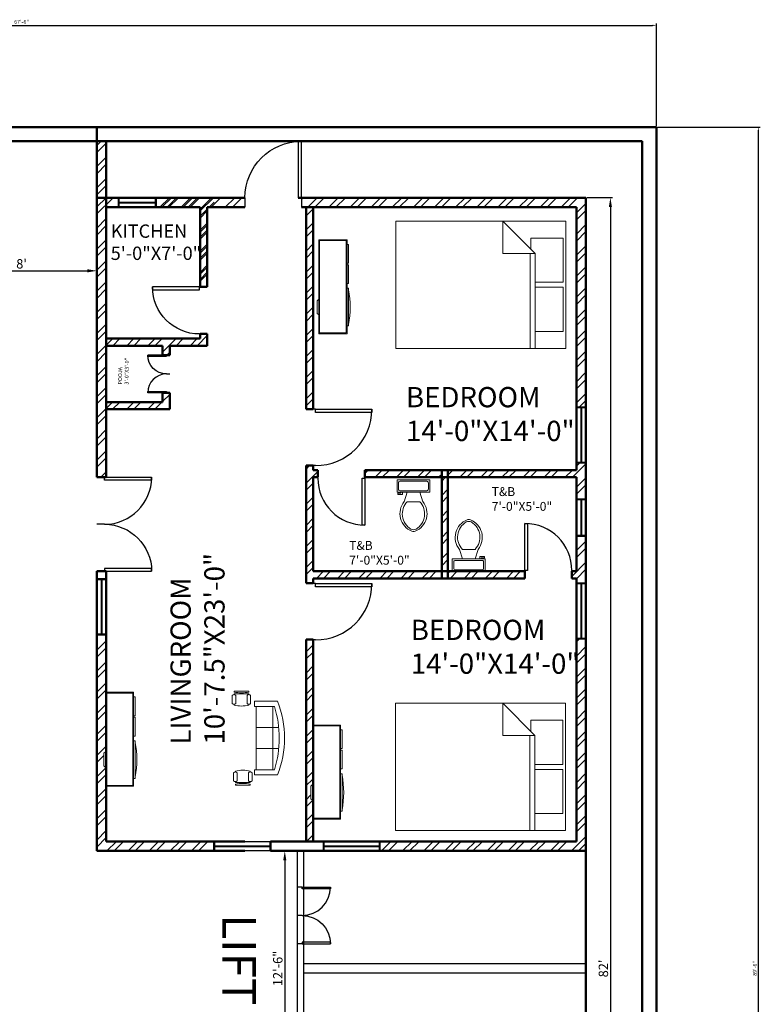
# Model space of a CAD drawing. Units: inches. Extents: x -12550 to 6516, y 1273 to 18700.
# Tile 19 of 19: x 6043 to 6516, y 1958 to 2587. Entities that reach past the tile are written whole.
import ezdxf

# ---------------------------------------------------------------- set-up
doc = ezdxf.new("R2010")
doc.units = ezdxf.units.IN
for name, color, linetype, lineweight in [('A-ANNO-DIMS', 2, 'Continuous', 18), ('A-AREA-IDEN', 1, 'Continuous', 18), ('A-DOOR', 5, 'Continuous', 25), ('A-EQPM', 4, 'Continuous', 25), ('A-FURN', 8, 'Continuous', 18), ('A-GLAZ', 3, 'Continuous', 25), ('A-WALL', 7, 'Continuous', 50), ('A-WALL-PATT', 8, 'Continuous', 13)]:
    doc.layers.add(name, color=color, linetype=linetype, lineweight=lineweight)
doc.styles.get("Standard").update_dxf_attribs({"font": 'arial.ttf'})
doc.dimstyles.new('ISO-25', dxfattribs={"dimtxt": 2.5, "dimasz": 2.5, "dimexe": 1.25, "dimexo": 0.625, "dimtad": 1, "dimlunit": 4, "dimtxsty": 'Standard', "dimcen": 2.5, "dimadec": 0, "dimazin": 0, "dimtfac": 1, "dimtmove": 0, "dimatfit": 3, "dimfxl": 1, "dimarcsym": 0})
pattern_1 = [(45, (3666.851, 0), (-6.735192, 6.735192), []), (45, (3671.341, 0), (-6.735192, 6.735192), [])]
pattern_2 = [(45, (3666.851, 567), (-6.735192, 6.735192), []), (45, (3671.341, 567), (-6.735192, 6.735192), [])]

# ---------------------------------------------------------------- blocks, each defined once
blk = doc.blocks.new('*U2')
for p, q in [((0, 0), (0, -5)), ((30, 0), (30, -5))]:
    blk.add_line(p, q)
blk.add_lwpolyline([(0, 0), (0, 30), (1.75, 30), (1.75, 0)], close=True)
blk.add_arc((0, 0), 30, 0, 90)
blk = doc.blocks.new('Bed - Queen')
for p, q in [((0, -80.00003), (0, 0)), ((0, 0), (59.99999, 0)), ((59.99999, 0), (59.99999, -80.00003)), ((7.99999, -1.2), (28.79998, -1.2)), ((7.99999, -14.4), (7.99999, -1.2)), ((28.79998, -1.2), (28.79998, -14.4)), ((31.19999, -1.2), (51.99999, -1.2)), ((31.19999, -14.4), (31.19999, -1.2)), ((51.99999, -1.2), (51.99999, -16.4)), ((0, -14.4), (44.8, -14.4)), ((44.8, -16.8), (0, -16.8)), ((59.99999, -29.6), (44.8, -14.4)), ((44.8, -14.4), (44.8, -29.6)), ((51.99999, -16.4), (46.79936, -16.4)), ((44.8, -29.6), (59.99999, -29.6)), ((59.99999, -80.00003), (0, -80.00003))]:
    blk.add_line(p, q)
blk = doc.blocks.new('Toilet - top')
for p, q in [((9.5, -6), (9.5, -2)), ((-10, -8.5), (-8, -8.5)), ((-10, -9.5), (-10, -8.5)), ((-7, -9.5), (-10, -9.5)), ((-8, -8.5), (-8, -8)), ((-7, -8), (-7, -9.5)), ((-4, -8), (-6, -14)), ((4, -8), (6, -14)), ((4, -14), (-4, -14))]:
    blk.add_line(p, q)
blk.add_lwpolyline([(10.5, -8), (10.5, 0), (-10.5, 0), (-10.5, -8)], close=True)
for points in [[(-9.5, -2), (-9.5, -6)], [(8.5, -1), (-8.5, -1)], [(-8.5, -7), (8.5, -7)]]:
    blk.add_lwpolyline(points)
for centre, radius, start, end in [((-8.62, -1.88), 0.884, 81.8699, 188.1301), ((-8.62, -6.12), 0.884, 171.8699, 278.1301), ((8.62, -1.88), 0.884, 351.8699, 98.1301), ((8.62, -6.12), 0.884, 261.8699, 8.1301), ((3.52, -21.58), 12.17, 141.46911, 247.97143), ((4.2, -21.82), 11.33, 136.36773, 238.94682), ((-3.52, -21.58), 12.17, 292.02843, 38.53071), ((-4.2, -21.82), 11.33, 301.05301, 43.63209), ((0, -27.88), 4, 245.73182, 294.26817), ((0, -29), 4, 254.86053, 285.13947)]:
    blk.add_arc(centre, radius, start, end)
blk = doc.blocks.new('Entertainment Center')
for p, q in [((-4, 0), (-5, -1)), ((4, 0), (-4, 0)), ((5, -1), (4, 0)), ((-17, -19), (-17, -1)), ((-17, -1), (43, -1)), ((-16.5, -18.5), (-16.5, -1.5)), ((-16.5, -1.5), (42.5, -1.5)), ((42.5, -1.5), (42.5, -18.5)), ((43, -1), (43, -19)), ((42.5, -18.5), (-16.5, -18.5)), ((43, -19), (-17, -19)), ((-12, -20), (-12, -19)), ((12, -20), (-12, -20)), ((12, -19), (12, -20)), ((15, -20), (15, -19)), ((27, -20), (15, -20)), ((27, -19), (27, -20)), ((28, -20), (28, -19)), ((40, -20), (28, -20)), ((40, -19), (40, -20))]:
    blk.add_line(p, q)
blk.add_arc((0, 40), 61, 259.6111, 280.3889)
blk = doc.blocks.new('Sofa - Roundback 7 ft.')
for p, q in [((-12.00002, -32.4421), (-12.00003, -6.5971)), ((11.99997, -32.4421), (11.99998, -6.5971)), ((-36.000027, -34), (-36.000027, -11.4696)), ((-35.999844, -13.3819), (35.9998, -13.3819)), ((35.99998, -34), (35.99998, -11.4696)), ((-36.000027, -32.4421), (35.99998, -32.4421))]:
    blk.add_line(p, q)
for points in [[(-36.000027, -34), (-42.000027, -34), (-42.000027, -8)], [(41.99998, -8), (41.99998, -34), (35.99998, -34)]]:
    blk.add_lwpolyline(points)
for centre, radius, start, end in [((0, -114.25), 114.25, 68.43141, 111.5686), ((-0.00001, -127.1968), 121.1968, 72.72033, 107.2797)]:
    blk.add_arc(centre, radius, start, end)
blk = doc.blocks.new('Chair - Desk')
for p, q in [((-8.5, 0), (-8.5, -1)), ((-8.5, 0), (8.5, 0)), ((8.5, 0), (8.5, -1)), ((-10.5, -5), (-10.5, -14)), ((-8.5, -3), (-8.5, -4)), ((-8.5, -3), (8.5, -3)), ((-6.5, -14), (-6.5, -5)), ((-2, -3), (-2, -1.9355)), ((2, -1.9576), (2, -3)), ((6.5, -5), (6.5, -14)), ((8.5, -3), (8.5, -4)), ((10.5, -14), (10.5, -5)), ((-8.5, -15), (-8.5, -16)), ((8.5, -15), (8.5, -16))]:
    blk.add_line(p, q)
for centre, radius, start, end in [((-8.5, -6.5), 2.5, 36.8699, 143.1301), ((0, 34.625), 36.625, 256.5803, 283.4197), ((8.5, -6.5), 2.5, 36.8699, 143.1301), ((-8.5, -12.5), 2.5, 216.8699, 323.1301), ((0, 19.625), 36.625, 256.5803, 283.4197), ((8.5, -12.5), 2.5, 216.8699, 323.1301)]:
    blk.add_arc(centre, radius, start, end)
blk = doc.blocks.new('*D52')
at = {"layer": 'A-ANNO-DIMS', "color": 0, "lineweight": -2, "transparency": 16777216}
for p, q in [((6219.91, 2056.25), (6211.2, 2056.25)), ((6212.45, 2050.25), (6212.45, 1912.25)), ((6219.91, 1906.25), (6211.2, 1906.25))]:
    blk.add_line(p, q, dxfattribs=at)
at = {"layer": 'A-ANNO-DIMS', "color": 0, "transparency": 16777216}
for points in [[(6211.45, 2050.25), (6213.45, 2050.25), (6212.45, 2056.25)], [(6211.45, 1912.25), (6213.45, 1912.25), (6212.45, 1906.25)]]:
    blk.add_solid(points, dxfattribs=at)
at = {"layer": 'Defpoints', "color": 0, "transparency": 16777216}
for p in [(6220.54, 2056.25), (6212.45, 1906.25), (6220.54, 1906.25)]:
    blk.add_point(p, dxfattribs=at)
at = {"layer": 'A-ANNO-DIMS', "color": 0, "transparency": 16777216, "insert": (6208.76, 1981.25), "char_height": 6, "attachment_point": 5, "rotation": 90}
blk.add_mtext('12\'-6"', dxfattribs=at)
blk = doc.blocks.new('*D54')
at = {"layer": 'A-ANNO-DIMS', "color": 0, "lineweight": -2, "transparency": 16777216}
for p, q in [((6405.16, 2473.25), (6421.41, 2473.25)), ((6420.16, 2467.25), (6420.16, 1495.25)), ((6405.16, 1489.25), (6421.41, 1489.25))]:
    blk.add_line(p, q, dxfattribs=at)
at = {"layer": 'A-ANNO-DIMS', "color": 0, "transparency": 16777216}
for points in [[(6419.16, 2467.25), (6421.16, 2467.25), (6420.16, 2473.25)], [(6419.16, 1495.25), (6421.16, 1495.25), (6420.16, 1489.25)]]:
    blk.add_solid(points, dxfattribs=at)
at = {"layer": 'Defpoints', "color": 0, "transparency": 16777216}
for p in [(6404.54, 2473.25), (6404.54, 1489.25), (6420.16, 1489.25)]:
    blk.add_point(p, dxfattribs=at)
at = {"layer": 'A-ANNO-DIMS', "color": 0, "transparency": 16777216, "insert": (6416.47, 1981.25), "char_height": 6, "attachment_point": 5, "rotation": 90}
blk.add_mtext("82'", dxfattribs=at)
blk = doc.blocks.new('*D51')
at = {"layer": 'A-ANNO-DIMS', "color": 0, "lineweight": -2, "transparency": 16777216}
for p, q in [((5996.54, 2407.12), (5996.54, 2427.81)), ((6002.54, 2426.56), (6086.54, 2426.56)), ((6092.54, 2407.12), (6092.54, 2427.81))]:
    blk.add_line(p, q, dxfattribs=at)
at = {"layer": 'A-ANNO-DIMS', "color": 0, "transparency": 16777216}
for points in [[(6002.54, 2427.56), (6002.54, 2425.56), (5996.54, 2426.56)], [(6086.54, 2427.56), (6086.54, 2425.56), (6092.54, 2426.56)]]:
    blk.add_solid(points, dxfattribs=at)
at = {"layer": 'Defpoints', "color": 0, "transparency": 16777216}
for p in [(6092.54, 2426.56), (5996.54, 2406.5), (6092.54, 2406.5)]:
    blk.add_point(p, dxfattribs=at)
at = {"layer": 'A-ANNO-DIMS', "color": 0, "transparency": 16777216, "insert": (6044.54, 2430.25), "char_height": 6, "attachment_point": 5}
blk.add_mtext("8'", dxfattribs=at)
blk = doc.blocks.new('WIN-3FT')
for p, q in [((0, 0), (0, 6)), ((0, 6), (36.02, 6)), ((36.02, 0), (0, 0)), ((0.5, 0), (0.5, 6)), ((35.52, 3.2), (0.5, 3.2)), ((35.52, 2.8), (0.5, 2.8)), ((35.52, 6), (35.52, 0)), ((36.02, 6), (36.02, 0))]:
    blk.add_line(p, q)
blk = doc.blocks.new('WIN-2FT')
for p, q in [((0, 0), (0, 24.02)), ((0, 24.02), (6, 24.02)), ((0, 23.52), (6, 23.52)), ((2.8, 0.5), (2.8, 23.52)), ((3.2, 0.5), (3.2, 23.52)), ((6, 24.02), (6, 0)), ((6, 0.5), (0, 0.5)), ((6, 0), (0, 0))]:
    blk.add_line(p, q)
blk = doc.blocks.new('*D121')
at = {"layer": 'A-ANNO-DIMS', "color": 0, "lineweight": -2, "transparency": 16777216}
for p, q in [((5639.54, 2518.87), (5639.54, 2584.5)), ((5642.04, 2583.25), (6447.04, 2583.25)), ((6449.54, 2518.87), (6449.54, 2584.5))]:
    blk.add_line(p, q, dxfattribs=at)
at = {"layer": 'A-ANNO-DIMS', "color": 0, "transparency": 16777216}
for points in [[(5642.04, 2583.66), (5642.04, 2582.83), (5639.54, 2583.25)], [(6447.04, 2583.66), (6447.04, 2582.83), (6449.54, 2583.25)]]:
    blk.add_solid(points, dxfattribs=at)
at = {"layer": 'Defpoints', "color": 0, "transparency": 16777216}
for p in [(6449.54, 2583.25), (5639.54, 2518.25), (6449.54, 2518.25)]:
    blk.add_point(p, dxfattribs=at)
at = {"layer": 'A-ANNO-DIMS', "color": 0, "transparency": 16777216, "insert": (6044.54, 2585.15), "char_height": 2.5, "attachment_point": 5}
blk.add_mtext('67\'-6"', dxfattribs=at)
blk = doc.blocks.new('*D122')
at = {"layer": 'A-ANNO-DIMS', "color": 0, "lineweight": -2, "transparency": 16777216}
for p, q in [((6450.16, 2518.25), (6515.79, 2518.25)), ((6514.54, 1446.75), (6514.54, 2515.75)), ((6450.16, 1444.25), (6515.79, 1444.25))]:
    blk.add_line(p, q, dxfattribs=at)
at = {"layer": 'A-ANNO-DIMS', "color": 0, "transparency": 16777216}
for points in [[(6514.12, 2515.75), (6514.96, 2515.75), (6514.54, 2518.25)], [(6514.12, 1446.75), (6514.96, 1446.75), (6514.54, 1444.25)]]:
    blk.add_solid(points, dxfattribs=at)
at = {"layer": 'Defpoints', "color": 0, "transparency": 16777216}
for p in [(6449.54, 2518.25), (6514.54, 2518.25), (6449.54, 1444.25)]:
    blk.add_point(p, dxfattribs=at)
at = {"layer": 'A-ANNO-DIMS', "color": 0, "transparency": 16777216, "insert": (6512.64, 1981.25), "char_height": 2.5, "attachment_point": 5, "rotation": 90}
blk.add_mtext('89\'-6"', dxfattribs=at)

msp = doc.modelspace()

# ---------------------------------------------------------------- hatches: boundary and pattern name
at = {"layer": 'A-WALL-PATT'}
h = msp.add_hatch(dxfattribs=at)
h.set_pattern_fill('ANSI32', color=256)
h.set_pattern_definition(pattern_1)
h.paths.add_polyline_path([(6098.54, 2509.247), (6092.54, 2509.247), (6092.54, 2473.247), (6098.54, 2473.247)])
h = msp.add_hatch(dxfattribs=at)
h.set_pattern_fill('ANSI32', color=256)
h.set_pattern_definition(pattern_2)
h.paths.add_polyline_path([(6106.297, 2473.247), (6092.54, 2473.247), (6092.54, 2294.747), (6097.54, 2294.747), (6098.54, 2294.747), (6098.54, 2467.247), (6106.297, 2467.247)])
h = msp.add_hatch(dxfattribs=at)
h.set_pattern_fill('ANSI32', color=256)
h.set_pattern_definition(pattern_1)
h.paths.add_polyline_path([(6130.314, 2473.247), (6130.314, 2467.247), (6158.54, 2467.247), (6158.54, 2416.247), (6163.04, 2416.247), (6163.04, 2467.247), (6187.04, 2467.247), (6187.04, 2473.247)])
h = msp.add_hatch(dxfattribs=at)
h.set_pattern_fill('ANSI32', color=256)
h.set_pattern_definition(pattern_2)
h.paths.add_polyline_path([(6167.378, 2473.247), (6130.314, 2473.247), (6130.314, 2467.247), (6158.54, 2467.247), (6158.54, 2416.247), (6163.04, 2416.247), (6163.04, 2467.247), (6167.378, 2467.247)])
h = msp.add_hatch(dxfattribs=at)
h.set_pattern_fill('ANSI32', color=256)
h.set_pattern_definition(pattern_2)
h.paths.add_polyline_path([(6223.04, 2473.247), (6223.04, 2467.247), (6398.54, 2467.247), (6398.54, 2339.747), (6404.54, 2339.747), (6404.54, 2473.247)])
h = msp.add_hatch(dxfattribs=at)
h.set_pattern_fill('ANSI32', color=256)
h.set_pattern_definition(pattern_2)
h.paths.add_polyline_path([(6230.54, 2467.247), (6226.04, 2467.247), (6226.04, 2338.247), (6230.54, 2338.247)])
h = msp.add_hatch(dxfattribs=at)
h.set_pattern_fill('ANSI32', color=256)
h.set_pattern_definition(pattern_2)
h.paths.add_polyline_path([(6163.04, 2386.247), (6158.54, 2386.247), (6158.54, 2383.247), (6098.54, 2383.247), (6098.54, 2378.747), (6134.54, 2378.747), (6134.54, 2372.747), (6137.04, 2372.747), (6139.04, 2372.747), (6139.04, 2378.747), (6163.04, 2378.747)])
h = msp.add_hatch(dxfattribs=at)
h.set_pattern_fill('ANSI32', color=256)
h.set_pattern_definition(pattern_2)
h.paths.add_polyline_path([(6139.04, 2348.747), (6137.04, 2348.747), (6134.54, 2348.747), (6134.54, 2342.747), (6098.54, 2342.747), (6098.54, 2338.247), (6139.04, 2338.247)])
h = msp.add_hatch(dxfattribs=at)
h.set_pattern_fill('ANSI32', color=256)
h.set_pattern_definition(pattern_2)
h.paths.add_polyline_path([(6230.54, 2294.747), (6233.54, 2294.747), (6233.54, 2299.247), (6230.54, 2299.247), (6230.54, 2302.247), (6226.04, 2302.247), (6226.04, 2227.247), (6230.54, 2227.247), (6230.54, 2230.247), (6233.492, 2230.247), (6312.54, 2230.247), (6312.54, 2234.747), (6233.492, 2234.747), (6230.54, 2234.747)])
h = msp.add_hatch(dxfattribs=at)
h.set_pattern_fill('ANSI32', color=256)
h.set_pattern_definition(pattern_2)
h.paths.add_polyline_path([(6404.54, 2303.73), (6398.54, 2303.73), (6398.54, 2299.247), (6395.54, 2299.247), (6316.54, 2299.247), (6316.54, 2294.747), (6395.54, 2294.747), (6398.54, 2294.747), (6398.54, 2281.042), (6404.54, 2281.042)])
h = msp.add_hatch(dxfattribs=at)
h.set_pattern_fill('ANSI32', color=256)
h.set_pattern_definition(pattern_2)
h.paths.add_polyline_path([(6312.54, 2299.247), (6263.54, 2299.247), (6263.54, 2294.747), (6312.54, 2294.747)], flags=17)
h = msp.add_hatch(dxfattribs=at)
h.set_pattern_fill('ANSI32', color=256)
h.set_pattern_definition(pattern_2)
h.paths.add_polyline_path([(6316.54, 2294.747), (6312.54, 2294.747), (6312.54, 2234.747), (6316.54, 2234.747)])
h = msp.add_hatch(dxfattribs=at)
h.set_pattern_fill('ANSI32', color=256)
h.set_pattern_definition(pattern_2)
h.paths.add_polyline_path([(6404.54, 2257.024), (6398.54, 2257.024), (6398.54, 2234.747), (6395.54, 2234.747), (6395.54, 2230.247), (6398.54, 2230.247), (6398.54, 2227.369), (6404.54, 2227.369)])
h = msp.add_hatch(dxfattribs=at)
h.set_pattern_fill('ANSI32', color=256)
h.set_pattern_definition(pattern_2)
h.paths.add_polyline_path([(6365.54, 2234.747), (6316.54, 2234.747), (6316.54, 2230.247), (6365.54, 2230.247)])
h = msp.add_hatch(dxfattribs=at)
h.set_pattern_fill('ANSI32', color=256)
h.set_pattern_definition(pattern_2)
h.paths.add_polyline_path([(6167.378, 2056.247), (6167.378, 2062.247), (6098.54, 2062.247), (6098.54, 2097.559), (6098.04, 2097.559), (6098.04, 2109.559), (6097.04, 2110.559), (6097.04, 2118.559), (6098.04, 2119.559), (6098.04, 2157.559), (6098.54, 2157.559), (6098.54, 2194.032), (6092.54, 2194.032), (6092.54, 2056.247)])
h = msp.add_hatch(dxfattribs=at)
h.set_pattern_fill('ANSI32', color=256)
h.set_pattern_definition(pattern_2)
h.paths.add_polyline_path([(6226.04, 2190.947), (6226.04, 2062.247), (6230.54, 2062.247), (6230.54, 2076.575), (6230.04, 2076.575), (6230.04, 2088.575), (6229.04, 2089.575), (6229.04, 2097.575), (6230.04, 2098.575), (6230.04, 2136.575), (6230.537, 2190.947)])
h = msp.add_hatch(dxfattribs=at)
h.set_pattern_fill('ANSI32', color=256)
h.set_pattern_definition(pattern_2)
h.paths.add_polyline_path([(6404.54, 2191.352), (6398.54, 2191.352), (6398.54, 2062.247), (6273.126, 2062.247), (6273.126, 2056.247), (6404.54, 2056.247)])

# ---------------------------------------------------------------- linework, layer by layer
at = {"layer": 'A-EQPM'}
for p, q in [((6220.54, 1906.247), (6220.54, 2056.247)), ((6404.54, 2056.247), (6220.54, 2056.247)), ((6224.54, 1906.247), (6224.54, 2056.247)), ((6404.54, 2056.247), (6404.54, 1906.247)), ((6404.54, 1984.247), (6224.54, 1984.247)), ((6404.54, 1978.247), (6224.54, 1978.247))]:
    msp.add_line(p, q, dxfattribs=at)
at = {"layer": 'A-WALL'}
for p, q in [((5639.54, 2518.247), (6449.54, 2518.247)), ((6092.54, 2294.747), (6092.54, 2518.247)), ((6449.54, 2518.247), (6449.54, 1444.247)), ((5648.54, 2509.247), (6440.54, 2509.247)), ((6220.94, 2509.247), (5920.94, 2509.247)), ((6098.54, 2294.747), (6098.54, 2509.247)), ((6440.54, 2509.247), (6440.54, 1453.247)), ((6187.04, 2473.247), (6092.54, 2473.247)), ((6226.04, 2473.247), (6220.94, 2473.247)), ((6404.54, 2473.247), (6226.04, 2473.247)), ((6404.54, 2060.923), (6404.54, 2473.247)), ((6158.54, 2467.247), (6098.54, 2467.247)), ((6158.54, 2416.247), (6158.54, 2467.247)), ((6187.04, 2467.247), (6163.04, 2467.247)), ((6163.04, 2416.247), (6163.04, 2467.247)), ((6226.04, 2467.247), (6223.04, 2467.247)), ((6398.54, 2467.247), (6226.04, 2467.247)), ((6226.04, 2338.247), (6226.04, 2467.247)), ((6230.54, 2338.247), (6230.54, 2467.247)), ((6398.54, 2299.247), (6398.54, 2467.247)), ((6158.54, 2416.247), (6163.04, 2416.247)), ((6158.54, 2383.247), (6098.54, 2383.247)), ((6158.54, 2383.247), (6158.54, 2386.247)), ((6163.04, 2386.247), (6158.54, 2386.247)), ((6163.04, 2378.747), (6163.04, 2386.247)), ((6163.04, 2383.247), (6163.04, 2386.247)), ((6134.54, 2378.747), (6098.54, 2378.747)), ((6134.54, 2372.747), (6134.54, 2378.747)), ((6163.04, 2378.747), (6139.04, 2378.747)), ((6139.04, 2372.747), (6139.04, 2378.747)), ((6134.54, 2372.747), (6139.04, 2372.747)), ((6134.54, 2342.747), (6134.54, 2348.747)), ((6139.04, 2348.747), (6134.54, 2348.747)), ((6139.04, 2338.247), (6139.04, 2348.747)), ((6139.04, 2342.747), (6139.04, 2348.747)), ((6134.54, 2342.747), (6098.54, 2342.747)), ((6139.04, 2338.247), (6098.54, 2338.247)), ((6226.04, 2338.247), (6230.54, 2338.247)), ((6226.04, 2227.247), (6226.04, 2302.247)), ((6230.54, 2302.247), (6226.04, 2302.247)), ((6230.54, 2299.247), (6230.54, 2302.247)), ((6230.54, 2299.247), (6230.54, 2302.247)), ((6230.54, 2299.247), (6230.54, 2302.247)), ((6230.54, 2299.247), (6230.54, 2302.247)), ((6098.54, 2294.747), (6092.54, 2294.747)), ((6233.54, 2299.247), (6230.54, 2299.247)), ((6233.54, 2294.747), (6230.54, 2294.747)), ((6230.54, 2234.747), (6230.54, 2294.747)), ((6230.54, 2234.747), (6230.54, 2294.747)), ((6230.54, 2234.747), (6230.54, 2294.747)), ((6230.54, 2294.747), (6233.54, 2294.747)), ((6233.54, 2294.747), (6233.54, 2299.247)), ((6395.54, 2299.247), (6263.54, 2299.247)), ((6263.54, 2299.247), (6263.54, 2294.747)), ((6395.54, 2294.747), (6263.54, 2294.747)), ((6312.54, 2230.247), (6312.54, 2299.247)), ((6316.54, 2230.247), (6316.54, 2299.247)), ((6398.54, 2299.247), (6395.54, 2299.247)), ((6398.54, 2299.247), (6395.54, 2299.247)), ((6398.54, 2294.747), (6395.54, 2294.747)), ((6398.54, 2234.747), (6398.54, 2294.747)), ((6098.54, 2234.747), (6092.54, 2234.747)), ((6092.54, 2056.247), (6092.54, 2234.747)), ((6098.54, 2062.247), (6098.54, 2234.747)), ((6233.492, 2234.747), (6230.54, 2234.747)), ((6365.54, 2234.747), (6233.492, 2234.747)), ((6365.54, 2234.747), (6365.54, 2230.247)), ((6398.54, 2234.747), (6395.54, 2234.747)), ((6395.54, 2230.247), (6395.54, 2234.747)), ((6226.04, 2230.247), (6226.04, 2227.247)), ((6226.04, 2227.247), (6230.54, 2227.247)), ((6233.492, 2230.247), (6230.54, 2230.247)), ((6230.54, 2227.247), (6230.54, 2230.247)), ((6230.54, 2227.247), (6230.54, 2230.247)), ((6230.54, 2227.247), (6230.54, 2230.247)), ((6365.54, 2230.247), (6233.492, 2230.247)), ((6398.54, 2230.247), (6395.54, 2230.247)), ((6398.54, 2230.247), (6395.54, 2230.247)), ((6398.54, 2062.247), (6398.54, 2230.247)), ((6226.04, 2062.247), (6226.04, 2191.247)), ((6230.54, 2191.247), (6226.04, 2191.247)), ((6230.54, 2062.247), (6230.54, 2191.247)), ((6187.04, 2062.247), (6098.54, 2062.247)), ((6167.378, 2062.247), (6167.378, 2056.247)), ((6203.396, 2062.247), (6203.396, 2056.247)), ((6223.04, 2062.247), (6203.396, 2062.247)), ((6398.54, 2062.247), (6223.04, 2062.247)), ((6226.04, 2062.247), (6223.04, 2062.247)), ((6187.04, 2056.247), (6092.54, 2056.247)), ((6203.396, 2056.247), (6223.04, 2056.247)), ((6404.54, 2056.247), (6223.04, 2056.247)), ((6404.54, 1489.247), (6404.54, 2060.923)), ((6440.54, 1489.247), (6440.54, 2060.923))]:
    msp.add_line(p, q, dxfattribs=at)

# ---------------------------------------------------------------- block references
at = {"layer": 'A-DOOR', "xscale": -1.199999999999999, "yscale": 1.199999999999999, "zscale": 1.199999999999999}
msp.add_blockref('*U2', (6223.04, 2473.247), dxfattribs=at)
at = {"layer": 'A-DOOR', "xscale": -1}
for p, rotation in [((6158.04, 2416.247), 90), ((6097.54, 2234.747), 270)]:
    msp.add_blockref('*U2', p, dxfattribs=dict(at, rotation=rotation))
at = {"layer": 'A-DOOR'}
for p, xscale, yscale, zscale, rotation in [((6137.04, 2372.747), -0.399999999999997, 0.399999999999997, 0.399999999999997, 90), ((6137.04, 2348.747), 0.399999999999997, 0.399999999999997, 0.399999999999997, 90.00000000000003), ((6232.04, 2338.247), 1.199999999999999, 1.199999999999999, 1.199999999999999, 270), ((6232.04, 2226.947), 1.199999999999999, 1.199999999999999, 1.199999999999999, 270)]:
    msp.add_blockref('*U2', p, dxfattribs=dict(at, xscale=xscale, yscale=yscale, zscale=zscale, rotation=rotation))
for p, rotation in [((6097.54, 2294.747), 270), ((6263.54, 2294.247), 180)]:
    msp.add_blockref('*U2', p, dxfattribs=dict(at, rotation=rotation))
msp.add_blockref('*U2', (6365.54, 2235.247), dxfattribs=at)
at = {"layer": 'A-EQPM', "yscale": 0.5999999999999954, "zscale": 0.5999999999999954, "rotation": 270}
for p, xscale in [((6223.54, 2033.042), 0.5999999999999954), ((6223.54, 1997.042), -0.5999999999999954)]:
    msp.add_blockref('*U2', p, dxfattribs=dict(at, xscale=xscale))
at = {"layer": 'A-FURN'}
for name, p, xscale, yscale, zscale, rotation in [('Bed - Queen', (6391.719, 2376.994), -1.354827908062564, 1.354827908062564, 1.354827908062564, 270), ('Sofa - Roundback 7 ft.', (6212.259, 2128.265), 0.5595223685495907, 0.5595223685495907, 0.5595223685495907, 270), ('Bed - Queen', (6391.559, 2069.217), -1.354827908062564, 1.354827908062564, 1.354827908062564, 270), ('Chair - Desk', (6185.673, 2098.281), 0.5595223685495907, 0.5595223685495907, 0.5595223685495907, 180)]:
    msp.add_blockref(name, p, dxfattribs=dict(at, xscale=xscale, yscale=yscale, zscale=zscale, rotation=rotation))
for name, p, rotation in [('Entertainment Center', (6233.169, 2403.379), 89.99999999999999), ('Toilet - top', (6329.808, 2234.747), 180), ('Entertainment Center', (6097.04, 2114.559), 89.99999999999999), ('Entertainment Center', (6229.04, 2093.575), 89.99999999999999)]:
    msp.add_blockref(name, p, dxfattribs=dict(at, rotation=rotation))
msp.add_blockref('Toilet - top', (6294.562, 2293.198), dxfattribs=at)
at = {"layer": 'A-FURN', "xscale": 0.5595223685495907, "yscale": 0.5595223685495907, "zscale": 0.5595223685495907}
msp.add_blockref('Chair - Desk', (6184.819, 2158.265), dxfattribs=at)
at = {"layer": 'A-GLAZ'}
for name, p, rotation in [('WIN-2FT', (6106.296, 2473.247), 269.9999999999974), ('WIN-3FT', (6404.54, 2303.73), 89.9999999999965), ('WIN-2FT', (6404.539, 2281.042), 180), ('WIN-3FT', (6098.54, 2194.032), 90.00000000000468), ('WIN-3FT', (6404.54, 2191.352), 89.99999999999625), ('WIN-3FT', (6203.395, 2062.247), 180), ('WIN-3FT', (6273.125, 2062.247), 180)]:
    msp.add_blockref(name, p, dxfattribs=dict(at, rotation=rotation))

# ---------------------------------------------------------------- texts
at = {"layer": 'A-AREA-IDEN', "attachment_point": 1}
for s, width, gutter_width, insert, char_height in [('KITCHEN\\P5\'-0"X7\'-0"', 1.29487, 42.422, (6101.42, 2456.124), 8.48435), ('T&B\\P7\'-0"X5\'-0"', 4.19569, 28.328, (6344.462, 2288.465), 5.66556), ('T&B\\P7\'-0"X5\'-0"', 4.19569, 28.328, (6253.552, 2254.107), 5.66556)]:
    msp.add_mtext_dynamic_manual_height_columns(s, width=width, gutter_width=gutter_width, heights=[0], dxfattribs=dict(at, insert=insert, char_height=char_height))
for s, width, gutter_width, insert, char_height, rotation in [('POOJA\\P3\'-0"X3\'-0"', 0.78585, 12.5, (6106.092, 2354.026), 2.5, 89.183853), ('LIFT', 3.27433, 107.272, (6194.027, 2015.823), 21.4543, 270)]:
    msp.add_mtext_dynamic_manual_height_columns(s, width=width, gutter_width=gutter_width, heights=[0], dxfattribs=dict(at, insert=insert, char_height=char_height, rotation=rotation))
at = {"layer": 'A-AREA-IDEN', "char_height": 12.93169, "attachment_point": 1}
for insert in [(6289.755, 2352.378), (6292.82, 2203.812)]:
    msp.add_mtext('BEDROOM\\P14\'-0"X14\'-0"', dxfattribs=dict(at, insert=insert))
at = {"layer": 'A-AREA-IDEN', "insert": (6139.563, 2124.153), "char_height": 12.93169, "attachment_point": 1, "rotation": 90}
msp.add_mtext('LIVINGROOM\\P10\'-7.5"X23\'-0"', dxfattribs=at)

# ---------------------------------------------------------------- dimensions: what is measured, and where the dimension line sits
at = {"layer": 'A-ANNO-DIMS'}
for base, p1, p2, override, picture, middle in [((6449.54, 2583.247), (5639.54, 2518.247), (6449.54, 2518.247), {"dimdec": 1, "dimlfac": 1, "dimrnd": 0, "dimzin": 1, "dimdsep": 46, "dimlunit": 4, "dimfrac": 2}, '*D121', (6044.54, 2585.149)), ((6092.54, 2426.562), (5996.54, 2406.497), (6092.54, 2406.497), {"dimtxt": 6, "dimasz": 6, "dimclrd": 0, "dimclre": 0, "dimclrt": 0}, '*D51', (6044.54, 2430.25))]:
    dim = msp.add_linear_dim(base=base, p1=p1, p2=p2, dimstyle='ISO-25', override=override, dxfattribs=at)
    dim.commit()
    dim.dimension.update_dxf_attribs({"geometry": picture, "text_midpoint": middle})
for base, p1, p2, override, picture, middle in [((6514.54, 2518.247), (6449.54, 1444.247), (6449.54, 2518.247), {"dimdec": 1, "dimlfac": 1, "dimrnd": 0, "dimzin": 1, "dimdsep": 46, "dimlunit": 4, "dimfrac": 2}, '*D122', (6512.638, 1981.247)), ((6420.159, 1489.247), (6404.54, 2473.247), (6404.54, 1489.247), {"dimtxt": 6, "dimasz": 6, "dimclrd": 0, "dimclre": 0, "dimclrt": 0}, '*D54', (6416.471, 1981.247)), ((6212.453, 1906.247), (6220.54, 2056.247), (6220.54, 1906.247), {"dimtxt": 6, "dimasz": 6, "dimclrd": 0, "dimclre": 0, "dimclrt": 0}, '*D52', (6208.764, 1981.247))]:
    dim = msp.add_linear_dim(base=base, p1=p1, p2=p2, angle=90, dimstyle='ISO-25', override=override, dxfattribs=at)
    dim.commit()
    dim.dimension.update_dxf_attribs({"geometry": picture, "text_midpoint": middle})

doc.saveas('drawing.dxf')
